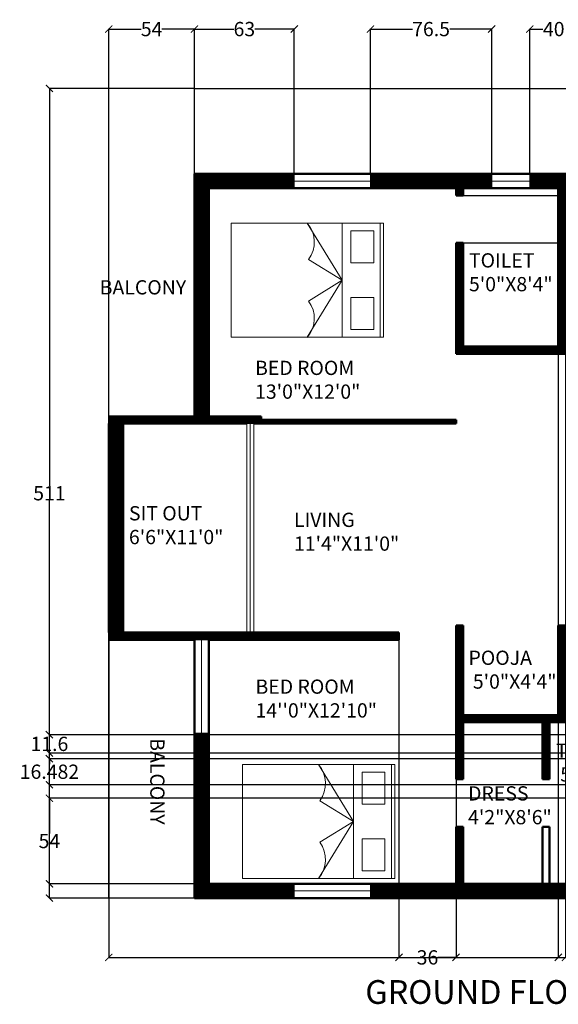
# Model space of a CAD drawing. Units: inches. Extents: x 273 to 1105, y 406 to 1027.
# Tile 1 of 3: x 273 to 612, y 406 to 1027. Entities that reach past the tile are written whole.
import ezdxf

# ---------------------------------------------------------------- set-up
doc = ezdxf.new("R2010")
doc.units = ezdxf.units.IN
doc.header["$MEASUREMENT"] = 0
for name, color, linetype, lineweight in [('A-ANNO-DIMS', 2, 'Continuous', 18), ('A-ANNO-TEXT', 7, 'Continuous', 25), ('A-AREA-IDEN', 7, 'Continuous', 18), ('A-FLOR-OTLN', 7, 'Continuous', 25), ('A-FURN', 8, 'Continuous', 18), ('A-GLAZ', 4, 'Continuous', 18), ('A-WALL', 7, 'Continuous', 50), ('A-WALL-PATT', 252, 'Continuous', 13)]:
    doc.layers.add(name, color=color, linetype=linetype, lineweight=lineweight)
doc.styles.get("Standard").update_dxf_attribs({"font": 'arial.ttf'})
doc.dimstyles.get("Standard").update_dxf_attribs({"dimtxt": 9, "dimasz": 4.5, "dimexe": 0.18, "dimexo": 0.0625, "dimgap": 0.09, "dimtad": 0, "dimtih": 1, "dimtoh": 1, "dimdec": 1, "dimzin": 0, "dimdsep": 46, "dimlunit": 4, "dimtxsty": 'Standard', "dimblk": 'ARCHTICK', "dimcen": 0.09, "dimadec": 0, "dimazin": 0, "dimtfac": 1, "dimtdec": 1, "dimtofl": 0, "dimtmove": 0, "dimatfit": 3, "dimfxl": 1, "dimtolj": 1, "dimtzin": 0, "dimarcsym": 0})

# ---------------------------------------------------------------- blocks, each defined once
blk = doc.blocks.new('BED-DOUBLE-72x96')
for p, q in [((0, 0.12), (0, 72.12)), ((0, 72.12), (96, 72.12)), ((48, 72.12), (70, 36.12)), ((70, 72.12), (70, 0.12)), ((94, 72.12), (94, 0.12)), ((96, 72.12), (96, 0.12)), ((48.84, 49.19), (70, 36.12)), ((70, 36.12), (48, 0.12)), ((70, 36.12), (48.84, 22.93)), ((96, 0.12), (0, 0.12))]:
    blk.add_line(p, q)
for points in [[(75.45, 67.24), (89.85, 67.24), (89.85, 47.07), (75.45, 47.07)], [(75.45, 5), (89.85, 5), (89.85, 25.18), (75.45, 25.18)]]:
    blk.add_lwpolyline(points, close=True)
for centre, start, end in [((33.83, 60.12), 323.92972, 40.25189), ((33.83, 12), 319.74811, 36.07028)]:
    blk.add_arc(centre, 18.57, start, end)
blk = doc.blocks.new('WIN-48')
for p, q in [((0, 9), (48, 9)), ((0, 0), (0, 9)), ((48, 9), (48, 0)), ((0, 4.5), (48, 4.5)), ((48, 0), (0, 0))]:
    blk.add_line(p, q)
blk = doc.blocks.new('WIN-24')
for p, q in [((0, 9), (24, 9)), ((0, 0), (0, 9)), ((24, 9), (24, 0)), ((0, 4.5), (24, 4.5)), ((24, 0), (0, 0))]:
    blk.add_line(p, q)
blk = doc.blocks.new('_ArchTick')
at = {"color": 0, "linetype": 'ByBlock', "const_width": 0.15}
blk.add_lwpolyline([(-0.5, -0.5), (0.5, 0.5)], dxfattribs=at)
blk = doc.blocks.new('*D14')
at = {"layer": 'A-ANNO-DIMS', "color": 0, "lineweight": -2, "transparency": 16777216}
for p, q in [((328.87, 472.54), (328.87, 434.97)), ((1048.37, 472.54), (1048.37, 434.97)), ((328.87, 435.15), (673.35, 435.15)), ((1048.37, 435.15), (703.9, 435.15))]:
    blk.add_line(p, q, dxfattribs=at)
at = {"layer": 'Defpoints', "color": 0, "transparency": 16777216}
for p in [(328.87, 472.6), (1048.37, 472.6), (1048.37, 435.15)]:
    blk.add_point(p, dxfattribs=at)
at = {"layer": 'A-ANNO-DIMS', "color": 0, "lineweight": -2, "transparency": 16777216, "xscale": 4.5, "yscale": 4.5, "zscale": 4.5, "rotation": 180}
blk.add_blockref('_ArchTick', (328.87, 435.15), dxfattribs=at)
at = {"layer": 'A-ANNO-DIMS', "color": 0, "lineweight": -2, "transparency": 16777216, "xscale": 4.5, "yscale": 4.5, "zscale": 4.5}
blk.add_blockref('_ArchTick', (1048.37, 435.15), dxfattribs=at)
at = {"layer": 'A-ANNO-DIMS', "color": 0, "transparency": 16777216, "insert": (688.62, 435.15), "char_height": 9, "attachment_point": 5}
blk.add_mtext('\\A1;719.5', dxfattribs=at)
blk = doc.blocks.new('*D15')
at = {"layer": 'A-ANNO-DIMS', "color": 0, "lineweight": -2, "transparency": 16777216}
for p, q in [((328.81, 983.6), (291.24, 983.6)), ((291.42, 983.6), (291.42, 732.79)), ((291.42, 472.6), (291.42, 723.42)), ((328.81, 472.6), (291.24, 472.6))]:
    blk.add_line(p, q, dxfattribs=at)
at = {"layer": 'Defpoints', "color": 0, "transparency": 16777216}
for p in [(291.42, 983.6), (328.87, 983.6), (328.87, 472.6)]:
    blk.add_point(p, dxfattribs=at)
at = {"layer": 'A-ANNO-DIMS', "color": 0, "lineweight": -2, "transparency": 16777216, "xscale": 4.5, "yscale": 4.5, "zscale": 4.5}
for p, rotation in [((291.42, 983.6), 90), ((291.42, 472.6), 270)]:
    blk.add_blockref('_ArchTick', p, dxfattribs=dict(at, rotation=rotation))
at = {"layer": 'A-ANNO-DIMS', "color": 0, "transparency": 16777216, "insert": (291.42, 728.1), "char_height": 9, "attachment_point": 5}
blk.add_mtext('\\A1;511', dxfattribs=at)
blk = doc.blocks.new('*D16')
at = {"layer": 'A-ANNO-DIMS', "color": 0, "lineweight": -2, "transparency": 16777216}
for p, q in [((328.87, 983.67), (328.87, 1021.23)), ((328.87, 1021.05), (349.36, 1021.05)), ((382.87, 1021.05), (362.39, 1021.05)), ((382.87, 929.67), (382.87, 1021.23))]:
    blk.add_line(p, q, dxfattribs=at)
at = {"layer": 'Defpoints', "color": 0, "transparency": 16777216}
for p in [(382.87, 1021.05), (328.87, 983.6), (382.87, 929.6)]:
    blk.add_point(p, dxfattribs=at)
at = {"layer": 'A-ANNO-DIMS', "color": 0, "lineweight": -2, "transparency": 16777216, "xscale": 4.5, "yscale": 4.5, "zscale": 4.5, "rotation": 180}
blk.add_blockref('_ArchTick', (328.87, 1021.05), dxfattribs=at)
at = {"layer": 'A-ANNO-DIMS', "color": 0, "lineweight": -2, "transparency": 16777216, "xscale": 4.5, "yscale": 4.5, "zscale": 4.5}
blk.add_blockref('_ArchTick', (382.87, 1021.05), dxfattribs=at)
at = {"layer": 'A-ANNO-DIMS', "color": 0, "transparency": 16777216, "insert": (355.87, 1021.05), "char_height": 9, "attachment_point": 5}
blk.add_mtext('\\A1;54', dxfattribs=at)
blk = doc.blocks.new('*D17')
at = {"layer": 'A-ANNO-DIMS', "color": 0, "lineweight": -2, "transparency": 16777216}
for p, q in [((382.87, 929.67), (382.87, 1021.23)), ((382.87, 1021.05), (407.81, 1021.05)), ((445.87, 1021.05), (420.93, 1021.05)), ((445.87, 929.67), (445.87, 1021.23))]:
    blk.add_line(p, q, dxfattribs=at)
at = {"layer": 'Defpoints', "color": 0, "transparency": 16777216}
for p in [(445.87, 1021.05), (382.87, 929.6), (445.87, 929.6)]:
    blk.add_point(p, dxfattribs=at)
at = {"layer": 'A-ANNO-DIMS', "color": 0, "lineweight": -2, "transparency": 16777216, "xscale": 4.5, "yscale": 4.5, "zscale": 4.5, "rotation": 180}
blk.add_blockref('_ArchTick', (382.87, 1021.05), dxfattribs=at)
at = {"layer": 'A-ANNO-DIMS', "color": 0, "lineweight": -2, "transparency": 16777216, "xscale": 4.5, "yscale": 4.5, "zscale": 4.5}
blk.add_blockref('_ArchTick', (445.87, 1021.05), dxfattribs=at)
at = {"layer": 'A-ANNO-DIMS', "color": 0, "transparency": 16777216, "insert": (414.37, 1021.05), "char_height": 9, "attachment_point": 5}
blk.add_mtext('\\A1;63', dxfattribs=at)
blk = doc.blocks.new('*D18')
at = {"layer": 'A-ANNO-DIMS', "color": 0, "lineweight": -2, "transparency": 16777216}
for p, q in [((493.87, 929.67), (493.87, 1021.23)), ((493.87, 1021.05), (520.35, 1021.05)), ((570.37, 1021.05), (543.9, 1021.05)), ((570.37, 929.67), (570.37, 1021.23))]:
    blk.add_line(p, q, dxfattribs=at)
at = {"layer": 'Defpoints', "color": 0, "transparency": 16777216}
for p in [(570.37, 1021.05), (493.87, 929.6), (570.37, 929.6)]:
    blk.add_point(p, dxfattribs=at)
at = {"layer": 'A-ANNO-DIMS', "color": 0, "lineweight": -2, "transparency": 16777216, "xscale": 4.5, "yscale": 4.5, "zscale": 4.5, "rotation": 180}
blk.add_blockref('_ArchTick', (493.87, 1021.05), dxfattribs=at)
at = {"layer": 'A-ANNO-DIMS', "color": 0, "lineweight": -2, "transparency": 16777216, "xscale": 4.5, "yscale": 4.5, "zscale": 4.5}
blk.add_blockref('_ArchTick', (570.37, 1021.05), dxfattribs=at)
at = {"layer": 'A-ANNO-DIMS', "color": 0, "transparency": 16777216, "insert": (532.12, 1021.05), "char_height": 9, "attachment_point": 5}
blk.add_mtext('\\A1;76.5', dxfattribs=at)
blk = doc.blocks.new('*D19')
at = {"layer": 'A-ANNO-DIMS', "color": 0, "lineweight": -2, "transparency": 16777216}
for p, q in [((594.37, 929.67), (594.37, 1021.23)), ((594.37, 1021.05), (602.63, 1021.05)), ((634.87, 1021.05), (626.62, 1021.05)), ((634.87, 929.67), (634.87, 1021.23))]:
    blk.add_line(p, q, dxfattribs=at)
at = {"layer": 'Defpoints', "color": 0, "transparency": 16777216}
for p in [(634.87, 1021.05), (594.37, 929.6), (634.87, 929.6)]:
    blk.add_point(p, dxfattribs=at)
at = {"layer": 'A-ANNO-DIMS', "color": 0, "lineweight": -2, "transparency": 16777216, "xscale": 4.5, "yscale": 4.5, "zscale": 4.5, "rotation": 180}
blk.add_blockref('_ArchTick', (594.37, 1021.05), dxfattribs=at)
at = {"layer": 'A-ANNO-DIMS', "color": 0, "lineweight": -2, "transparency": 16777216, "xscale": 4.5, "yscale": 4.5, "zscale": 4.5}
blk.add_blockref('_ArchTick', (634.87, 1021.05), dxfattribs=at)
at = {"layer": 'A-ANNO-DIMS', "color": 0, "transparency": 16777216, "insert": (614.62, 1021.05), "char_height": 9, "attachment_point": 5}
blk.add_mtext('\\A1;40.5', dxfattribs=at)
blk = doc.blocks.new('*D27')
at = {"layer": 'A-ANNO-DIMS', "color": 0, "lineweight": -2, "transparency": 16777216}
for p, q in [((825.31, 535.6), (291.24, 535.6)), ((291.42, 535.6), (291.42, 513.27)), ((291.42, 481.6), (291.42, 503.94)), ((825.31, 481.6), (291.24, 481.6))]:
    blk.add_line(p, q, dxfattribs=at)
at = {"layer": 'Defpoints', "color": 0, "transparency": 16777216}
for p in [(291.42, 535.6), (825.37, 535.6), (825.37, 481.6)]:
    blk.add_point(p, dxfattribs=at)
at = {"layer": 'A-ANNO-DIMS', "color": 0, "lineweight": -2, "transparency": 16777216, "xscale": 4.5, "yscale": 4.5, "zscale": 4.5}
for p, rotation in [((291.42, 535.6), 90), ((291.42, 481.6), 270)]:
    blk.add_blockref('_ArchTick', p, dxfattribs=dict(at, rotation=rotation))
at = {"layer": 'A-ANNO-DIMS', "color": 0, "transparency": 16777216, "insert": (291.42, 508.6), "char_height": 9, "attachment_point": 5}
blk.add_mtext('\\A1;54', dxfattribs=at)
blk = doc.blocks.new('*D30')
at = {"layer": 'A-ANNO-DIMS', "color": 0, "lineweight": -2, "transparency": 16777216}
for p, q in [((552.44, 916.1), (1086, 916.1)), ((1085.82, 916.1), (1085.82, 905.79)), ((1085.82, 886.1), (1085.82, 896.42)), ((552.44, 886.1), (1086, 886.1))]:
    blk.add_line(p, q, dxfattribs=at)
at = {"layer": 'Defpoints', "color": 0, "transparency": 16777216}
for p in [(552.37, 916.1), (552.37, 886.1), (1085.82, 886.1)]:
    blk.add_point(p, dxfattribs=at)
at = {"layer": 'A-ANNO-DIMS', "color": 0, "lineweight": -2, "transparency": 16777216, "xscale": 4.5, "yscale": 4.5, "zscale": 4.5}
for p, rotation in [((1085.82, 916.1), 90), ((1085.82, 886.1), 270)]:
    blk.add_blockref('_ArchTick', p, dxfattribs=dict(at, rotation=rotation))
at = {"layer": 'A-ANNO-DIMS', "color": 0, "transparency": 16777216, "insert": (1085.82, 901.1), "char_height": 9, "attachment_point": 5}
blk.add_mtext('\\A1;30', dxfattribs=at)
blk = doc.blocks.new('*D31')
at = {"layer": 'A-ANNO-DIMS', "color": 0, "lineweight": -2, "transparency": 16777216}
for p, q in [((612.37, 820.54), (612.37, 434.97)), ((616.87, 820.54), (616.87, 434.97)), ((612.37, 435.15), (616.87, 435.15)), ((616.87, 435.15), (621.37, 435.15))]:
    blk.add_line(p, q, dxfattribs=at)
at = {"layer": 'Defpoints', "color": 0, "transparency": 16777216}
for p in [(612.37, 820.6), (616.87, 820.6), (616.87, 435.15)]:
    blk.add_point(p, dxfattribs=at)
at = {"layer": 'A-ANNO-DIMS', "color": 0, "lineweight": -2, "transparency": 16777216, "xscale": 4.5, "yscale": 4.5, "zscale": 4.5, "rotation": 180}
blk.add_blockref('_ArchTick', (612.37, 435.15), dxfattribs=at)
at = {"layer": 'A-ANNO-DIMS', "color": 0, "lineweight": -2, "transparency": 16777216, "xscale": 4.5, "yscale": 4.5, "zscale": 4.5}
blk.add_blockref('_ArchTick', (616.87, 435.15), dxfattribs=at)
at = {"layer": 'A-ANNO-DIMS', "color": 0, "transparency": 16777216, "insert": (629.87, 435.15), "char_height": 9, "attachment_point": 5}
blk.add_mtext('\\A1;4.5', dxfattribs=at)
blk = doc.blocks.new('*D32')
at = {"layer": 'A-ANNO-DIMS', "color": 0, "lineweight": -2, "transparency": 16777216}
for p, q in [((511.87, 640.04), (511.87, 434.97)), ((547.87, 640.04), (547.87, 434.97)), ((511.87, 435.15), (523.34, 435.15)), ((547.87, 435.15), (536.4, 435.15))]:
    blk.add_line(p, q, dxfattribs=at)
at = {"layer": 'Defpoints', "color": 0, "transparency": 16777216}
for p in [(511.87, 640.1), (547.87, 640.1), (547.87, 435.15)]:
    blk.add_point(p, dxfattribs=at)
at = {"layer": 'A-ANNO-DIMS', "color": 0, "lineweight": -2, "transparency": 16777216, "xscale": 4.5, "yscale": 4.5, "zscale": 4.5, "rotation": 180}
blk.add_blockref('_ArchTick', (511.87, 435.15), dxfattribs=at)
at = {"layer": 'A-ANNO-DIMS', "color": 0, "lineweight": -2, "transparency": 16777216, "xscale": 4.5, "yscale": 4.5, "zscale": 4.5}
blk.add_blockref('_ArchTick', (547.87, 435.15), dxfattribs=at)
at = {"layer": 'A-ANNO-DIMS', "color": 0, "transparency": 16777216, "insert": (529.87, 435.15), "char_height": 9, "attachment_point": 5}
blk.add_mtext('\\A1;36', dxfattribs=at)
blk = doc.blocks.new('*D35')
at = {"layer": 'A-ANNO-DIMS', "color": 0, "lineweight": -2, "transparency": 16777216}
for p, q in [((717.55, 560.57), (291.24, 560.57)), ((291.42, 560.57), (291.42, 557.01)), ((291.42, 544.09), (291.42, 547.64)), ((717.55, 544.09), (291.24, 544.09))]:
    blk.add_line(p, q, dxfattribs=at)
at = {"layer": 'Defpoints', "color": 0, "transparency": 16777216}
for p in [(717.61, 560.57), (291.42, 544.09), (717.61, 544.09)]:
    blk.add_point(p, dxfattribs=at)
at = {"layer": 'A-ANNO-DIMS', "color": 0, "lineweight": -2, "transparency": 16777216, "xscale": 4.5, "yscale": 4.5, "zscale": 4.5}
for p, rotation in [((291.42, 560.57), 90), ((291.42, 544.09), 270)]:
    blk.add_blockref('_ArchTick', p, dxfattribs=dict(at, rotation=rotation))
at = {"layer": 'A-ANNO-DIMS', "color": 0, "transparency": 16777216, "insert": (291.42, 552.33), "char_height": 9, "attachment_point": 5}
blk.add_mtext('\\A1;16.482', dxfattribs=at)
blk = doc.blocks.new('*D39')
at = {"layer": 'A-ANNO-DIMS', "color": 0, "lineweight": -2, "transparency": 16777216}
for p, q in [((805.12, 575.7), (291.24, 575.7)), ((291.42, 575.7), (291.42, 574.59)), ((801.31, 564.1), (291.24, 564.1)), ((291.42, 564.1), (291.42, 565.22))]:
    blk.add_line(p, q, dxfattribs=at)
at = {"layer": 'Defpoints', "color": 0, "transparency": 16777216}
for p in [(291.42, 575.7), (805.18, 575.7), (801.37, 564.1)]:
    blk.add_point(p, dxfattribs=at)
at = {"layer": 'A-ANNO-DIMS', "color": 0, "lineweight": -2, "transparency": 16777216, "xscale": 4.5, "yscale": 4.5, "zscale": 4.5}
for p, rotation in [((291.42, 575.7), 90), ((291.42, 564.1), 270)]:
    blk.add_blockref('_ArchTick', p, dxfattribs=dict(at, rotation=rotation))
at = {"layer": 'A-ANNO-DIMS', "color": 0, "transparency": 16777216, "insert": (291.42, 569.9), "char_height": 9, "attachment_point": 5}
blk.add_mtext('\\A1;11.6', dxfattribs=at)

msp = doc.modelspace()

# ---------------------------------------------------------------- hatches: boundary and pattern name
at = {"layer": 'A-WALL-PATT'}
h = msp.add_hatch(dxfattribs=at)
h.set_pattern_fill('ANSI31', color=256)
h.paths.add_polyline_path([(735.2471, 481.6046), (681.3741, 481.6046), (681.3741, 535.6046), (825.3741, 535.6046), (825.3741, 481.6046), (783.2471, 481.6046), (783.2471, 472.6046), (834.3741, 472.6046), (834.3741, 592.6046), (861.3741, 592.6046), (861.3741, 601.6046), (834.3741, 601.6046), (834.3741, 721.6046), (918.3741, 721.6046), (918.3741, 601.6046), (891.3741, 601.6046), (891.3741, 592.6046), (960.3741, 592.6046), (960.3741, 617.3546), (951.3741, 617.3546), (951.3741, 601.6046), (927.3741, 601.6046), (927.3741, 657.1046), (951.3741, 657.1046), (951.3741, 641.3546), (960.3741, 641.3546), (960.3741, 681.8546), (951.3741, 681.8546), (951.3741, 666.1046), (927.3741, 666.1046), (927.3741, 721.6046), (951.3741, 721.6046), (951.3741, 705.8546), (960.3741, 705.8546), (960.3741, 727.1046), (834.3741, 727.1046), (825.3741, 727.1046), (825.3741, 640.1046), (681.3741, 640.1046), (676.8741, 640.1046), (676.8741, 635.6046), (681.3741, 635.6046), (825.3741, 635.6046), (825.3741, 540.1046), (681.3741, 540.1046), (681.3741, 588.1046), (676.8741, 588.1046), (616.8741, 588.1046), (616.8741, 644.6046), (612.3741, 644.6046), (612.3741, 640.1046), (612.3741, 588.1046), (552.3741, 588.1046), (552.3741, 640.1046), (552.3741, 644.6046), (547.8741, 644.6046), (547.8741, 640.1046), (547.8741, 635.6046), (547.8741, 547.6046), (552.3741, 547.6046), (552.3741, 583.6046), (602.3741, 583.6046), (602.3741, 547.6046), (606.8741, 547.6046), (606.8741, 583.6046), (676.8741, 583.6046), (676.8741, 481.6046), (552.3741, 481.6046), (552.3741, 517.6046), (547.8741, 517.6046), (547.8741, 481.6046), (493.8741, 481.6046), (493.8741, 472.6046), (547.8741, 472.6046), (735.2471, 472.6046)])
h.paths.add_polyline_path([(445.8741, 481.6046), (391.8741, 481.6046), (391.8741, 576.6354), (382.8741, 576.6354), (382.8741, 472.6046), (391.8741, 472.6046), (445.8741, 472.6046)])
h.paths.add_polyline_path([(729.3741, 929.6046), (658.8741, 929.6046), (658.8741, 920.6046), (676.8741, 920.6046), (676.8741, 916.1046), (681.3741, 916.1046), (681.3741, 920.6046), (729.3741, 920.6046)])
h.paths.add_polyline_path([(834.3741, 929.6046), (777.3741, 929.6046), (777.3741, 920.6046), (825.3741, 920.6046), (825.3741, 776.6046), (681.3741, 776.6046), (676.8741, 776.6046), (676.8741, 772.1046), (681.3741, 772.1046), (825.3741, 772.1046), (825.3741, 763.1046), (834.3741, 763.1046)])
h.paths.add_polyline_path([(1048.3741, 850.6046), (834.3741, 850.6046), (834.3741, 841.6046), (1048.3741, 841.6046)])
h.paths.add_polyline_path([(337.8741, 772.1046), (391.8741, 772.1046), (415.8741, 772.1046), (420.3741, 772.1046), (424.8741, 772.1046), (547.8741, 772.1046), (547.8741, 774.3546), (424.8741, 774.3546), (424.8741, 776.6046), (391.8741, 776.6046), (391.8741, 920.6046), (445.8741, 920.6046), (445.8741, 929.6046), (382.8741, 929.6046), (382.8741, 776.6046), (328.8741, 776.6046), (328.8741, 772.1046), (328.8741, 635.6046), (382.8741, 635.6046), (391.8741, 635.6046), (424.8741, 635.6046), (511.8741, 635.6046), (511.8741, 640.1046), (415.8741, 640.1046), (391.8741, 640.1046), (337.8741, 640.1046)])
h.paths.add_polyline_path([(570.3741, 929.6046), (493.8741, 929.6046), (493.8741, 920.6046), (547.8741, 920.6046), (547.8741, 916.1046), (552.3741, 916.1046), (552.3741, 920.6046), (570.3741, 920.6046)])
h.paths.add_polyline_path([(634.8741, 929.6046), (594.3741, 929.6046), (594.3741, 920.6046), (612.3741, 920.6046), (612.3741, 820.6046), (552.3741, 820.6046), (552.3741, 886.1046), (547.8741, 886.1046), (547.8741, 816.1046), (552.3741, 816.1046), (612.3741, 816.1046), (616.8741, 816.1046), (676.8741, 816.1046), (681.3741, 816.1046), (681.3741, 886.1046), (676.8741, 886.1046), (676.8741, 820.6046), (616.8741, 820.6046), (616.8741, 920.6046), (634.8741, 920.6046)])

# ---------------------------------------------------------------- linework, layer by layer
at = {"layer": 'A-FLOR-OTLN'}
for p, q in [((328.8741, 772.1046), (328.8741, 983.6046)), ((382.8741, 983.6046), (328.8741, 983.6046)), ((382.8741, 983.6046), (834.3741, 983.6046)), ((328.8741, 472.6046), (328.8741, 772.1046)), ((328.8741, 640.1046), (328.8741, 472.6046)), ((382.8741, 472.6046), (328.8741, 472.6046))]:
    msp.add_line(p, q, dxfattribs=at)
at = {"layer": 'A-GLAZ'}
for p, q in [((415.8741, 772.1046), (415.8741, 640.1046)), ((415.8741, 772.1046), (420.3741, 772.1046)), ((418.1241, 772.1046), (418.1241, 640.1046)), ((420.3741, 772.1046), (420.3741, 640.1046)), ((382.8741, 635.6046), (391.8741, 635.6046)), ((387.3741, 635.6046), (387.3741, 576.6354)), ((391.8741, 576.6354), (382.8741, 576.6354))]:
    msp.add_line(p, q, dxfattribs=at)
at = {"layer": 'A-WALL'}
for p, q in [((382.8741, 929.6046), (382.8741, 776.6046)), ((382.8741, 929.6046), (834.3741, 929.6046)), ((391.8741, 920.6046), (391.8741, 776.6046)), ((391.8741, 920.6046), (547.8741, 920.6046)), ((547.8741, 920.6046), (547.8741, 916.1046)), ((552.3741, 920.6046), (552.3741, 916.1046)), ((552.3741, 920.6046), (612.3741, 920.6046)), ((612.3741, 920.6046), (612.3741, 820.6046)), ((552.3741, 916.1046), (547.8741, 916.1046)), ((552.3741, 886.1046), (547.8741, 886.1046)), ((547.8741, 886.1046), (547.8741, 816.1046)), ((552.3741, 886.1046), (552.3741, 820.6046)), ((552.3741, 820.6046), (612.3741, 820.6046)), ((552.3741, 816.1046), (547.8741, 816.1046)), ((552.3741, 816.1046), (612.3741, 816.1046)), ((612.3741, 816.1046), (616.8741, 816.1046)), ((382.8741, 776.6046), (328.8741, 776.6046)), ((328.8741, 772.1046), (328.8741, 640.1046)), ((337.8741, 772.1046), (337.8741, 640.1046)), ((391.8741, 772.1046), (337.8741, 772.1046)), ((391.8741, 776.6046), (424.8741, 776.6046)), ((391.8741, 772.1046), (415.8741, 772.1046)), ((420.3741, 772.1046), (424.8741, 772.1046)), ((424.8741, 774.3546), (424.8741, 776.6046)), ((424.8741, 774.3546), (547.8741, 774.3546)), ((424.8741, 772.1046), (547.8741, 772.1046)), ((547.8741, 774.3546), (547.8741, 772.1046)), ((391.8741, 640.1046), (337.8741, 640.1046)), ((391.8741, 640.1046), (415.8741, 640.1046)), ((415.8741, 640.1046), (511.8741, 640.1046)), ((511.8741, 640.1046), (511.8741, 635.6046)), ((552.3741, 644.6046), (547.8741, 644.6046)), ((547.8741, 644.6046), (547.8741, 640.1046)), ((547.8741, 640.1046), (547.8741, 635.6046)), ((552.3741, 640.1046), (552.3741, 644.6046)), ((552.3741, 640.1046), (552.3741, 588.1046)), ((612.3741, 644.6046), (616.8741, 644.6046)), ((612.3741, 640.1046), (612.3741, 644.6046)), ((612.3741, 640.1046), (612.3741, 588.1046)), ((382.8741, 635.6046), (328.8741, 635.6046)), ((382.8741, 635.6046), (382.8741, 472.6046)), ((391.8741, 635.6046), (424.8741, 635.6046)), ((391.8741, 635.6046), (391.8741, 481.6046)), ((424.8741, 635.6046), (511.8741, 635.6046)), ((547.8741, 635.6046), (547.8741, 547.6046)), ((552.3741, 588.1046), (612.3741, 588.1046)), ((552.3741, 583.6046), (602.3741, 583.6046)), ((552.3741, 583.6046), (552.3741, 547.6046)), ((602.3741, 583.6046), (602.3741, 547.6046)), ((606.8741, 583.6046), (606.8741, 547.6046)), ((606.8741, 583.6046), (676.8741, 583.6046)), ((552.3741, 547.6046), (547.8741, 547.6046)), ((602.3741, 547.6046), (606.8741, 547.6046)), ((552.3741, 517.6046), (547.8741, 517.6046)), ((547.8741, 517.6046), (547.8741, 481.6046)), ((552.3741, 517.6046), (552.3741, 481.6046)), ((602.3741, 517.6046), (606.8741, 517.6046)), ((602.3741, 517.6046), (602.3741, 481.6046)), ((606.8741, 517.6046), (606.8741, 481.6046)), ((391.8741, 481.6046), (547.8741, 481.6046)), ((552.3741, 481.6046), (676.8741, 481.6046)), ((391.8741, 472.6046), (382.8741, 472.6046)), ((391.8741, 472.6046), (547.8741, 472.6046)), ((547.8741, 472.6046), (834.3741, 472.6046))]:
    msp.add_line(p, q, dxfattribs=at)

# ---------------------------------------------------------------- block references
at = {"layer": 'A-FURN'}
for p in [(406.0856, 826.452), (413.1793, 484.8693)]:
    msp.add_blockref('BED-DOUBLE-72x96', p, dxfattribs=at)
at = {"layer": 'A-GLAZ'}
for name, p in [('WIN-48', (445.874, 920.605)), ('WIN-24', (570.374, 920.605)), ('WIN-48', (445.874, 472.605))]:
    msp.add_blockref(name, p, dxfattribs=at)

# ---------------------------------------------------------------- texts
at = {"layer": 'A-ANNO-TEXT', "insert": (490.6396, 420.8046), "char_height": 15, "attachment_point": 1}
msp.add_mtext_dynamic_manual_height_columns('GROUND FLOOR PLAN', width=435.167248, gutter_width=1, heights=[0], dxfattribs=at)
at = {"layer": 'A-AREA-IDEN', "char_height": 9, "attachment_point": 1}
for s, insert in [(' TOILET\\P 5\'0"X8\'4"', (553.2856, 879.559)), ('BALCONY', (323.1236, 862.5496)), ('BED ROOM\\P13\'0"X12\'0"', (421.132, 811.7139)), (' SIT OUT\\P 6\'6"X11\'0"', (338.8251, 719.9493)), ('LIVING\\P11\'4"X11\'0"', (445.6736, 715.8019)), ('POOJA\\P 5\'0"X4\'4"', (555.7405, 628.7482)), ('BED ROOM\\P14\'\'0"X12\'10"', (421.3942, 610.5289)), ('TOILET\\P 5\'0"X8\'6"', (610.8677, 570.119)), ('  DRESS\\P  4\'2"X8\'6"', (549.9811, 543.1626))]:
    msp.add_mtext_dynamic_manual_height_columns(s, width=435.167248, gutter_width=1, heights=[0], dxfattribs=dict(at, insert=insert))
at = {"layer": 'A-AREA-IDEN', "insert": (364.0097, 573.4722), "char_height": 9, "attachment_point": 1, "rotation": 270}
msp.add_mtext_dynamic_manual_height_columns('BALCONY', width=435.167248, gutter_width=1, heights=[0], dxfattribs=at)

# ---------------------------------------------------------------- dimensions: what is measured, and where the dimension line sits
at = {"layer": 'A-ANNO-DIMS'}
for base, p1, p2, override, picture, middle in [((382.8741, 1021.0546), (328.8741, 983.6046), (382.8741, 929.6046), {"dimdec": 0, "dimlfac": 1, "dimrnd": 0, "dimzin": 0, "dimdsep": 46, "dimlunit": 2}, '*D16', (355.8741, 1021.0546)), ((445.8741, 1021.0546), (382.8741, 929.6046), (445.8741, 929.6046), {"dimdec": 0, "dimlfac": 1, "dimrnd": 0, "dimzin": 0, "dimdsep": 46, "dimlunit": 2}, '*D17', (414.3741, 1021.0546)), ((570.3741, 1021.0546), (493.8741, 929.6046), (570.3741, 929.6046), {"dimdec": 1, "dimlfac": 1, "dimrnd": 0, "dimzin": 0, "dimdsep": 46, "dimlunit": 2}, '*D18', (532.1241, 1021.0546)), ((634.8741, 1021.0546), (594.3741, 929.6046), (634.8741, 929.6046), {"dimdec": 1, "dimlfac": 1, "dimrnd": 0, "dimzin": 0, "dimdsep": 46, "dimlunit": 2}, '*D19', (614.6241, 1021.0546)), ((616.8741, 435.1546), (612.3741, 820.6046), (616.8741, 820.6046), {"dimdec": 1, "dimlfac": 1, "dimrnd": 0, "dimzin": 0, "dimdsep": 46, "dimlunit": 2}, '*D31', (629.8717, 435.1546)), ((547.8741, 435.1546), (511.8741, 640.1046), (547.8741, 640.1046), {"dimdec": 0, "dimlfac": 1, "dimrnd": 0, "dimzin": 0, "dimdsep": 46, "dimlunit": 2}, '*D32', (529.8741, 435.1546)), ((1048.3741, 435.1546), (328.8741, 472.6046), (1048.3741, 472.6046), {"dimdec": 1, "dimlfac": 1, "dimrnd": 0, "dimzin": 0, "dimdsep": 46, "dimlunit": 2}, '*D14', (688.6241, 435.1546))]:
    dim = msp.add_linear_dim(base=base, p1=p1, p2=p2, dimstyle='Standard', override=override, dxfattribs=at)
    dim.commit()
    dim.dimension.update_dxf_attribs({"geometry": picture, "text_midpoint": middle})
for base, p1, p2, override, picture, middle in [((291.4241, 983.6046), (328.8741, 472.6046), (328.8741, 983.6046), {"dimdec": 0, "dimlfac": 1, "dimrnd": 0, "dimzin": 0, "dimdsep": 46, "dimlunit": 2}, '*D15', (291.4241, 728.1046)), ((1085.8241, 886.1046), (552.3741, 916.1046), (552.3741, 886.1046), {"dimdec": 0, "dimlfac": 1, "dimrnd": 0, "dimzin": 0, "dimdsep": 46, "dimlunit": 2}, '*D30', (1085.8241, 901.1046)), ((291.4241, 575.7043), (801.3741, 564.1046), (805.1776, 575.7043), {"dimdec": 1, "dimlfac": 1, "dimrnd": 0, "dimzin": 0, "dimdsep": 46, "dimlunit": 2}, '*D39', (291.4241, 569.9045)), ((291.4241, 544.0857), (717.6111, 560.5674), (717.6111, 544.0857), {"dimdec": 3, "dimlfac": 1, "dimrnd": 0, "dimzin": 0, "dimdsep": 46, "dimlunit": 2}, '*D35', (291.4241, 552.3266)), ((291.4241, 535.6046), (825.3741, 481.6046), (825.3741, 535.6046), {"dimdec": 0, "dimlfac": 1, "dimrnd": 0, "dimzin": 0, "dimdsep": 46, "dimlunit": 2}, '*D27', (291.4241, 508.6046))]:
    dim = msp.add_linear_dim(base=base, p1=p1, p2=p2, angle=90, dimstyle='Standard', override=override, dxfattribs=at)
    dim.commit()
    dim.dimension.update_dxf_attribs({"geometry": picture, "text_midpoint": middle})

doc.saveas('drawing.dxf')
